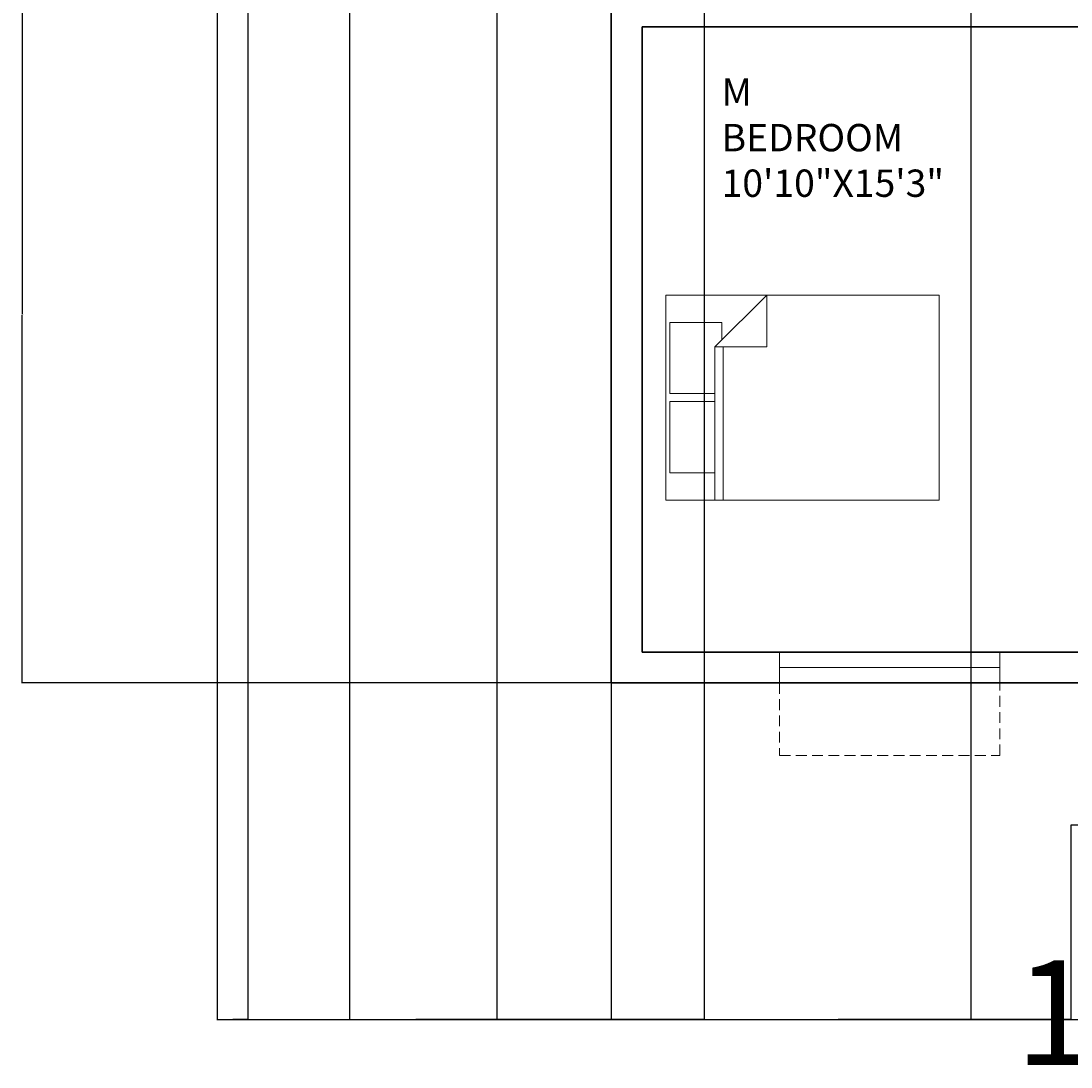
# Model space of a CAD drawing. Units: inches. Extents: x 276 to 912, y -567 to 621.
# Tile 1 of 7: x 276 to 583, y -567 to -261. Entities that reach past the tile are written whole.
import ezdxf

# ---------------------------------------------------------------- set-up
doc = ezdxf.new("R2010")
doc.units = ezdxf.units.IN
doc.linetypes.add('HIDDEN2', pattern=[4.7625, 3.175, -1.5875])
for name, color, linetype, lineweight in [('A-ANNO-DIMS', 2, 'Continuous', 18), ('A-ANNO-TEXT', 7, 'Continuous', 35), ('A-AREA-IDEN', 7, 'Continuous', 18), ('A-FLOR-OVHD', 8, 'HIDDEN2', 13), ('A-FURN', 8, 'Continuous', 18), ('A-GLAZ', 4, 'Continuous', 18), ('A-WALL', 7, 'Continuous', 35)]:
    doc.layers.add(name, color=color, linetype=linetype, lineweight=lineweight)
doc.dimstyles.get("Standard").update_dxf_attribs({"dimtxt": 0.18, "dimasz": 0.18, "dimexe": 0.18, "dimexo": 0.0625, "dimgap": 0.09, "dimtad": 0, "dimtih": 1, "dimtoh": 1, "dimdec": 4, "dimzin": 0, "dimdsep": 46, "dimtxsty": 'Standard', "dimcen": 0.09, "dimadec": 0, "dimazin": 0, "dimtfac": 1, "dimtdec": 4, "dimtofl": 0, "dimtmove": 0, "dimatfit": 3, "dimfxl": 1, "dimtolj": 1, "dimtzin": 0, "dimarcsym": 0})

# ---------------------------------------------------------------- blocks, each defined once
blk = doc.blocks.new('Bed - Queen')
for p, q in [((0, -80.00003), (0, 0)), ((0, 0), (59.99999, 0)), ((59.99999, 0), (59.99999, -80.00003)), ((7.99999, -1.2), (28.79998, -1.2)), ((7.99999, -14.4), (7.99999, -1.2)), ((28.79998, -1.2), (28.79998, -14.4)), ((31.19999, -1.2), (51.99999, -1.2)), ((31.19999, -14.4), (31.19999, -1.2)), ((51.99999, -1.2), (51.99999, -16.4)), ((0, -14.4), (44.8, -14.4)), ((59.99999, -29.6), (44.8, -14.4)), ((44.8, -14.4), (44.8, -29.6)), ((44.8, -16.8), (0, -16.8)), ((51.99999, -16.4), (46.79936, -16.4)), ((44.8, -29.6), (59.99999, -29.6)), ((59.99999, -80.00003), (0, -80.00003))]:
    blk.add_line(p, q)
blk = doc.blocks.new('*D24')
at = {"layer": 'A-ANNO-DIMS', "color": 0, "lineweight": -2, "transparency": 16777216}
for p, q in [((333.082179, 103.255751), (333.082179, -553.223061)), ((854.209085, -327.604004), (854.209085, -553.223061)), ((333.262179, -553.043061), (593.255632, -553.043061)), ((854.029085, -553.043061), (594.035632, -553.043061))]:
    blk.add_line(p, q, dxfattribs=at)
at = {"layer": 'A-ANNO-DIMS', "color": 0, "transparency": 16777216}
for points in [[(333.262179, -553.013061), (333.262179, -553.073061), (333.082179, -553.043061)], [(854.029085, -553.013061), (854.029085, -553.073061), (854.209085, -553.043061)]]:
    blk.add_solid(points, dxfattribs=at)
at = {"layer": 'Defpoints', "color": 0, "transparency": 16777216}
for p in [(333.082179, 103.318251), (854.209085, -327.541504), (854.209085, -553.043061)]:
    blk.add_point(p, dxfattribs=at)
at = {"layer": 'A-ANNO-DIMS', "color": 0, "transparency": 16777216, "insert": (593.645632, -553.043061), "char_height": 0.18, "attachment_point": 5}
blk.add_mtext('\\A1;521.1', dxfattribs=at)
blk = doc.blocks.new('*D25')
at = {"layer": 'A-ANNO-DIMS', "color": 0, "lineweight": -2, "transparency": 16777216}
for p, q in [((478.5, 564.29), (911.39, 564.29)), ((911.21, 564.11), (911.21, 34.31)), ((911.21, -495.86), (911.21, 33.95)), ((582.98, -496.04), (911.39, -496.04))]:
    blk.add_line(p, q, dxfattribs=at)
at = {"layer": 'A-ANNO-DIMS', "color": 0, "transparency": 16777216}
for points in [[(911.18, 564.11), (911.24, 564.11), (911.21, 564.29)], [(911.18, -495.86), (911.24, -495.86), (911.21, -496.04)]]:
    blk.add_solid(points, dxfattribs=at)
at = {"layer": 'Defpoints', "color": 0, "transparency": 16777216}
for p in [(478.44, 564.29), (582.92, -496.04), (911.21, -496.04)]:
    blk.add_point(p, dxfattribs=at)
at = {"layer": 'A-ANNO-DIMS', "color": 0, "transparency": 16777216, "insert": (911.21, 34.13), "char_height": 0.18, "attachment_point": 5}
blk.add_mtext('\\A1;1060.3', dxfattribs=at)
blk = doc.blocks.new('*D31')
at = {"layer": 'A-ANNO-DIMS', "color": 0, "lineweight": -2, "transparency": 16777216}
for p, q in [((333.082179, 103.255751), (333.082179, -553.223061)), ((475.582179, 65.246155), (475.582179, -553.223061)), ((333.262179, -553.043061), (403.912179, -553.043061)), ((475.402179, -553.043061), (404.752179, -553.043061))]:
    blk.add_line(p, q, dxfattribs=at)
at = {"layer": 'A-ANNO-DIMS', "color": 0, "transparency": 16777216}
for points in [[(333.262179, -553.013061), (333.262179, -553.073061), (333.082179, -553.043061)], [(475.402179, -553.013061), (475.402179, -553.073061), (475.582179, -553.043061)]]:
    blk.add_solid(points, dxfattribs=at)
at = {"layer": 'Defpoints', "color": 0, "transparency": 16777216}
for p in [(333.082179, 103.318251), (475.582179, 65.308655), (475.582179, -553.043061)]:
    blk.add_point(p, dxfattribs=at)
at = {"layer": 'A-ANNO-DIMS', "color": 0, "transparency": 16777216, "insert": (404.332179, -553.043061), "char_height": 0.18, "attachment_point": 5}
blk.add_mtext('\\A1;142.5', dxfattribs=at)
blk = doc.blocks.new('*D32')
at = {"layer": 'A-ANNO-DIMS', "color": 0, "lineweight": -2, "transparency": 16777216}
for p, q in [((475.582179, 65.246155), (475.582179, -553.223061)), ((553.582179, 65.246155), (553.582179, -553.223061)), ((475.762179, -553.043061), (514.342179, -553.043061)), ((553.402179, -553.043061), (514.822179, -553.043061))]:
    blk.add_line(p, q, dxfattribs=at)
at = {"layer": 'A-ANNO-DIMS', "color": 0, "transparency": 16777216}
for points in [[(475.762179, -553.013061), (475.762179, -553.073061), (475.582179, -553.043061)], [(553.402179, -553.013061), (553.402179, -553.073061), (553.582179, -553.043061)]]:
    blk.add_solid(points, dxfattribs=at)
at = {"layer": 'Defpoints', "color": 0, "transparency": 16777216}
for p in [(475.582179, 65.308655), (553.582179, 65.308655), (553.582179, -553.043061)]:
    blk.add_point(p, dxfattribs=at)
at = {"layer": 'A-ANNO-DIMS', "color": 0, "transparency": 16777216, "insert": (514.582179, -553.043061), "char_height": 0.18, "attachment_point": 5}
blk.add_mtext('\\A1;78', dxfattribs=at)
blk = doc.blocks.new('*D33')
at = {"layer": 'A-ANNO-DIMS', "color": 0, "lineweight": -2, "transparency": 16777216}
for p, q in [((553.582179, 65.246155), (553.582179, -553.223061)), ((668.582179, 65.246155), (668.582179, -553.223061)), ((553.762179, -553.043061), (610.812179, -553.043061)), ((668.402179, -553.043061), (611.352179, -553.043061))]:
    blk.add_line(p, q, dxfattribs=at)
at = {"layer": 'A-ANNO-DIMS', "color": 0, "transparency": 16777216}
for points in [[(553.762179, -553.013061), (553.762179, -553.073061), (553.582179, -553.043061)], [(668.402179, -553.013061), (668.402179, -553.073061), (668.582179, -553.043061)]]:
    blk.add_solid(points, dxfattribs=at)
at = {"layer": 'Defpoints', "color": 0, "transparency": 16777216}
for p in [(553.582179, 65.308655), (668.582179, 65.308655), (668.582179, -553.043061)]:
    blk.add_point(p, dxfattribs=at)
at = {"layer": 'A-ANNO-DIMS', "color": 0, "transparency": 16777216, "insert": (611.082179, -553.043061), "char_height": 0.18, "attachment_point": 5}
blk.add_mtext('\\A1;115', dxfattribs=at)
blk = doc.blocks.new('*D41')
at = {"layer": 'A-ANNO-DIMS', "color": 0, "lineweight": -2, "transparency": 16777216}
for p, q in [((333.082179, 363.769143), (333.082179, -553.223061)), ((342.082179, 363.769143), (342.082179, -553.223061)), ((333.262179, -553.043061), (337.432179, -553.043061)), ((341.902179, -553.043061), (337.732179, -553.043061))]:
    blk.add_line(p, q, dxfattribs=at)
at = {"layer": 'A-ANNO-DIMS', "color": 0, "transparency": 16777216}
for points in [[(333.262179, -553.013061), (333.262179, -553.073061), (333.082179, -553.043061)], [(341.902179, -553.013061), (341.902179, -553.073061), (342.082179, -553.043061)]]:
    blk.add_solid(points, dxfattribs=at)
at = {"layer": 'Defpoints', "color": 0, "transparency": 16777216}
for p in [(333.082179, 363.831643), (342.082179, 363.831643), (342.082179, -553.043061)]:
    blk.add_point(p, dxfattribs=at)
at = {"layer": 'A-ANNO-DIMS', "color": 0, "transparency": 16777216, "insert": (337.582179, -553.043061), "char_height": 0.18, "attachment_point": 5}
blk.add_mtext('\\A1;9', dxfattribs=at)
blk = doc.blocks.new('*D55')
at = {"layer": 'A-ANNO-DIMS', "color": 0, "lineweight": -2, "transparency": 16777216}
for p, q in [((333.082179, -239.052429), (333.082179, -553.223061)), ((448.418489, -454.604004), (448.418489, -553.223061)), ((333.262179, -553.043061), (390.270334, -553.043061)), ((448.238489, -553.043061), (391.230334, -553.043061))]:
    blk.add_line(p, q, dxfattribs=at)
at = {"layer": 'A-ANNO-DIMS', "color": 0, "transparency": 16777216}
for points in [[(333.262179, -553.013061), (333.262179, -553.073061), (333.082179, -553.043061)], [(448.238489, -553.013061), (448.238489, -553.073061), (448.418489, -553.043061)]]:
    blk.add_solid(points, dxfattribs=at)
at = {"layer": 'Defpoints', "color": 0, "transparency": 16777216}
for p in [(333.082179, -238.989929), (448.418489, -454.541504), (448.418489, -553.043061)]:
    blk.add_point(p, dxfattribs=at)
at = {"layer": 'A-ANNO-DIMS', "color": 0, "transparency": 16777216, "insert": (390.750334, -553.043061), "char_height": 0.18, "attachment_point": 5}
blk.add_mtext('\\A1;115.34', dxfattribs=at)
blk = doc.blocks.new('*D56')
at = {"layer": 'A-ANNO-DIMS', "color": 0, "lineweight": -2, "transparency": 16777216}
for p, q in [((448.418489, -454.604004), (448.418489, -553.223061)), ((582.918489, -496.105561), (582.918489, -553.223061)), ((448.598489, -553.043061), (515.248489, -553.043061)), ((582.738489, -553.043061), (516.088489, -553.043061))]:
    blk.add_line(p, q, dxfattribs=at)
at = {"layer": 'A-ANNO-DIMS', "color": 0, "transparency": 16777216}
for points in [[(448.598489, -553.013061), (448.598489, -553.073061), (448.418489, -553.043061)], [(582.738489, -553.013061), (582.738489, -553.073061), (582.918489, -553.043061)]]:
    blk.add_solid(points, dxfattribs=at)
at = {"layer": 'Defpoints', "color": 0, "transparency": 16777216}
for p in [(448.418489, -454.541504), (582.918489, -496.043061), (582.918489, -553.043061)]:
    blk.add_point(p, dxfattribs=at)
at = {"layer": 'A-ANNO-DIMS', "color": 0, "transparency": 16777216, "insert": (515.668489, -553.043061), "char_height": 0.18, "attachment_point": 5}
blk.add_mtext('\\A1;134.5', dxfattribs=at)
blk = doc.blocks.new('*D57')
at = {"layer": 'A-ANNO-DIMS', "color": 0, "lineweight": -2, "transparency": 16777216}
for p, q in [((582.918489, -496.105561), (582.918489, -553.223061)), ((660.918489, -496.105561), (660.918489, -553.223061)), ((583.098489, -553.043061), (621.678489, -553.043061)), ((660.738489, -553.043061), (622.158489, -553.043061))]:
    blk.add_line(p, q, dxfattribs=at)
at = {"layer": 'A-ANNO-DIMS', "color": 0, "transparency": 16777216}
for points in [[(583.098489, -553.013061), (583.098489, -553.073061), (582.918489, -553.043061)], [(660.738489, -553.013061), (660.738489, -553.073061), (660.918489, -553.043061)]]:
    blk.add_solid(points, dxfattribs=at)
at = {"layer": 'Defpoints', "color": 0, "transparency": 16777216}
for p in [(582.918489, -496.043061), (660.918489, -496.043061), (660.918489, -553.043061)]:
    blk.add_point(p, dxfattribs=at)
at = {"layer": 'A-ANNO-DIMS', "color": 0, "transparency": 16777216, "insert": (621.918489, -553.043061), "char_height": 0.18, "attachment_point": 5}
blk.add_mtext('\\A1;78', dxfattribs=at)
blk = doc.blocks.new('*D64')
at = {"layer": 'A-ANNO-DIMS', "color": 0, "lineweight": -2, "transparency": 16777216}
for p, q in [((371.772434, -239.052429), (371.772434, -553.223061)), ((414.936626, -239.052429), (414.936626, -553.223061)), ((371.952434, -553.043061), (392.93453, -553.043061)), ((414.756626, -553.043061), (393.77453, -553.043061))]:
    blk.add_line(p, q, dxfattribs=at)
at = {"layer": 'A-ANNO-DIMS', "color": 0, "transparency": 16777216}
for points in [[(371.952434, -553.013061), (371.952434, -553.073061), (371.772434, -553.043061)], [(414.756626, -553.013061), (414.756626, -553.073061), (414.936626, -553.043061)]]:
    blk.add_solid(points, dxfattribs=at)
at = {"layer": 'Defpoints', "color": 0, "transparency": 16777216}
for p in [(371.772434, -238.989929), (414.936626, -238.989929), (414.936626, -553.043061)]:
    blk.add_point(p, dxfattribs=at)
at = {"layer": 'A-ANNO-DIMS', "color": 0, "transparency": 16777216, "insert": (393.35453, -553.043061), "char_height": 0.18, "attachment_point": 5}
blk.add_mtext('\\A1;43.16', dxfattribs=at)
blk = doc.blocks.new('*D75')
at = {"layer": 'A-ANNO-DIMS', "color": 0, "lineweight": -2, "transparency": 16777216}
for p, q in [((448.36, -238.99), (275.9, -238.99)), ((276.08, -239.17), (276.08, -346.59)), ((276.08, -454.36), (276.08, -346.95)), ((448.36, -454.54), (275.9, -454.54))]:
    blk.add_line(p, q, dxfattribs=at)
at = {"layer": 'A-ANNO-DIMS', "color": 0, "transparency": 16777216}
for points in [[(276.05, -239.17), (276.11, -239.17), (276.08, -238.99)], [(276.05, -454.36), (276.11, -454.36), (276.08, -454.54)]]:
    blk.add_solid(points, dxfattribs=at)
at = {"layer": 'Defpoints', "color": 0, "transparency": 16777216}
for p in [(276.08, -238.99), (448.42, -238.99), (448.42, -454.54)]:
    blk.add_point(p, dxfattribs=at)
at = {"layer": 'A-ANNO-DIMS', "color": 0, "transparency": 16777216, "insert": (276.08, -346.77), "char_height": 0.18, "attachment_point": 5}
blk.add_mtext('\\A1;215.55', dxfattribs=at)

msp = doc.modelspace()

# ---------------------------------------------------------------- linework, layer by layer
at = {"layer": 'A-FLOR-OVHD'}
for p, q in [((497.6447, -454.5415), (497.6447, -475.7843)), ((562.0976, -475.7843), (562.0976, -454.5415)), ((497.6447, -475.7843), (562.0976, -475.7843))]:
    msp.add_line(p, q, dxfattribs=at)
at = {"layer": 'A-GLAZ'}
for p, q in [((497.6447, -450.0415), (497.6447, -445.5415)), ((497.6447, -445.5415), (497.6447, -454.5415)), ((562.0976, -445.5415), (562.0976, -454.5415)), ((562.0976, -450.0415), (497.6447, -450.0415)), ((562.0976, -454.5415), (562.0976, -450.0415))]:
    msp.add_line(p, q, dxfattribs=at)
at = {"layer": 'A-WALL'}
for p, q in [((448.4185, -238.9899), (448.4185, -454.5415)), ((457.4185, -262.5415), (592.4185, -262.5415)), ((457.4185, -262.5415), (457.4185, -445.5415)), ((457.4185, -445.5415), (587.4185, -445.5415)), ((457.4185, -454.5415), (448.4185, -454.5415)), ((457.4185, -454.5415), (812.9185, -454.5415))]:
    msp.add_line(p, q, dxfattribs=at)

# ---------------------------------------------------------------- block references
at = {"layer": 'A-FURN', "rotation": 90}
msp.add_blockref('Bed - Queen', (464.3523, -401.0298), dxfattribs=at)

# ---------------------------------------------------------------- texts
at = {"layer": 'A-ANNO-TEXT', "insert": (566.519, -535.6866), "char_height": 30.703761, "attachment_point": 1}
msp.add_mtext_dynamic_manual_height_columns('{\\fTimes New Roman|b0|i0|c0|p18;1262SFT}', width=239.005817, gutter_width=47.9746, heights=[0], dxfattribs=at)
at = {"layer": 'A-AREA-IDEN', "insert": (480.6977, -277.6436), "char_height": 8, "attachment_point": 1}
msp.add_mtext_dynamic_manual_height_columns('{\\fTimes New Roman|b0|i0|c0|p18;M BEDROOM\\P10\'10"X15\'3"}', width=62.274017, gutter_width=12.5, heights=[0], dxfattribs=at)

# ---------------------------------------------------------------- dimensions: what is measured, and where the dimension line sits
at = {"layer": 'A-ANNO-DIMS'}
for base, p1, p2, override, picture, middle in [((911.2091, -496.0431), (478.4357, 564.2937), (582.9185, -496.0431), {"dimdec": 1, "dimlfac": 1, "dimrnd": 0, "dimzin": 0, "dimdsep": 46, "dimlunit": 2}, '*D25', (911.2091, 34.1253)), ((276.0822, -238.9899), (448.4185, -454.5415), (448.4185, -238.9899), {"dimdec": 2, "dimlfac": 1, "dimrnd": 0, "dimzin": 0, "dimdsep": 46, "dimlunit": 2}, '*D75', (276.0822, -346.7657))]:
    dim = msp.add_linear_dim(base=base, p1=p1, p2=p2, angle=90, dimstyle='Standard', override=override, dxfattribs=at)
    dim.commit()
    dim.dimension.update_dxf_attribs({"geometry": picture, "text_midpoint": middle})
for base, p1, p2, override, picture, middle in [((342.0822, -553.0431), (333.0822, 363.8316), (342.0822, 363.8316), {"dimdec": 0, "dimlfac": 1, "dimrnd": 0, "dimzin": 0, "dimdsep": 46, "dimlunit": 2}, '*D41', (337.5822, -553.0431)), ((854.2091, -553.0431), (333.0822, 103.3183), (854.2091, -327.5415), {"dimdec": 1, "dimlfac": 1, "dimrnd": 0, "dimzin": 0, "dimdsep": 46, "dimlunit": 2}, '*D24', (593.6456, -553.0431)), ((475.5822, -553.0431), (333.0822, 103.3183), (475.5822, 65.3087), {"dimdec": 1, "dimlfac": 1, "dimrnd": 0, "dimzin": 0, "dimdsep": 46, "dimlunit": 2}, '*D31', (404.3322, -553.0431)), ((553.5822, -553.0431), (475.5822, 65.3087), (553.5822, 65.3087), {"dimdec": 0, "dimlfac": 1, "dimrnd": 0, "dimzin": 0, "dimdsep": 46, "dimlunit": 2}, '*D32', (514.5822, -553.0431)), ((668.5822, -553.0431), (553.5822, 65.3087), (668.5822, 65.3087), {"dimdec": 0, "dimlfac": 1, "dimrnd": 0, "dimzin": 0, "dimdsep": 46, "dimlunit": 2}, '*D33', (611.0822, -553.0431)), ((448.4185, -553.0431), (333.0822, -238.9899), (448.4185, -454.5415), {"dimdec": 2, "dimlfac": 1, "dimrnd": 0, "dimzin": 0, "dimdsep": 46, "dimlunit": 2}, '*D55', (390.7503, -553.0431)), ((414.9366, -553.0431), (371.7724, -238.9899), (414.9366, -238.9899), {"dimdec": 2, "dimlfac": 1, "dimrnd": 0, "dimzin": 0, "dimdsep": 46, "dimlunit": 2}, '*D64', (393.3545, -553.0431)), ((582.9185, -553.0431), (448.4185, -454.5415), (582.9185, -496.0431), {"dimdec": 1, "dimlfac": 1, "dimrnd": 0, "dimzin": 0, "dimdsep": 46, "dimlunit": 2}, '*D56', (515.6685, -553.0431)), ((660.9185, -553.0431), (582.9185, -496.0431), (660.9185, -496.0431), {"dimdec": 0, "dimlfac": 1, "dimrnd": 0, "dimzin": 0, "dimdsep": 46, "dimlunit": 2}, '*D57', (621.9185, -553.0431))]:
    dim = msp.add_linear_dim(base=base, p1=p1, p2=p2, dimstyle='Standard', override=override, dxfattribs=at)
    dim.commit()
    dim.dimension.update_dxf_attribs({"geometry": picture, "text_midpoint": middle})

doc.saveas('drawing.dxf')
